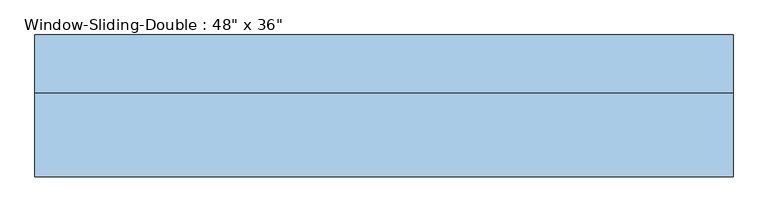
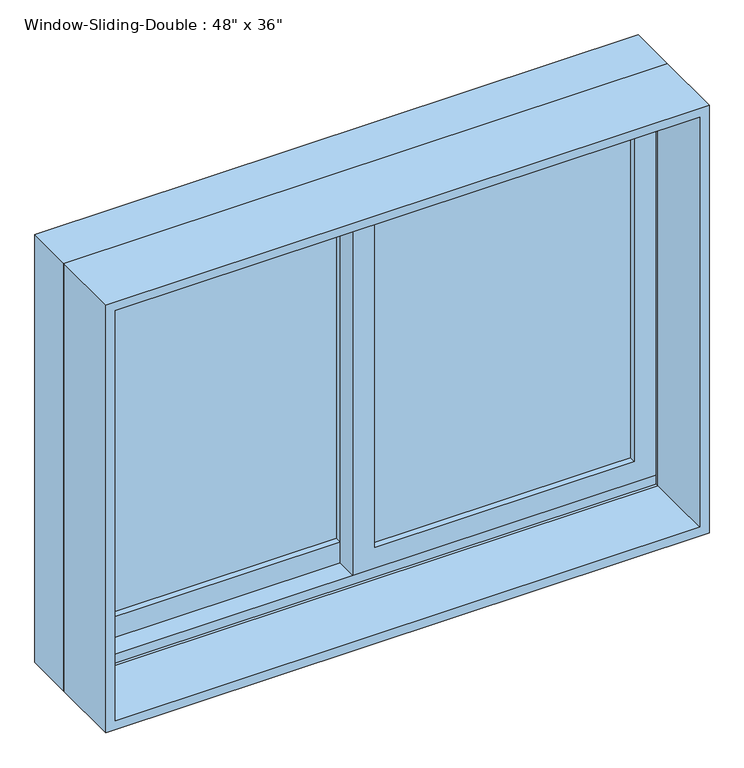
"""IFC4 building model written with IfcOpenShell, lengths in millimetres: window geometry."""

from ifc_helpers import new_model, si_unit, frame, origin, place, context, project, spatial, polyline, outline, extrude, faceted_brep, source, transform, mapped, element, save


def window_2eef0573(model_context):
    return source(origin(), model_context, "Body", "SolidModel", [
        extrude(outline(polyline([(952.5, 590.55), (1809.75, 590.55), (1809.75, -22.225), (952.5, -22.225), (952.5, 590.55)]), holes=[polyline([(996.95, 22.225), (1765.3, 22.225), (1765.3, 546.1), (996.95, 546.1), (996.95, 22.225)])]), frame((0.0, 34.29, 0.0), z_axis=(0.0, 1.0, 0.0), x_axis=(0.0, 0.0, 1.0)), (0.0, 0.0, 1.0), 44.45),
        extrude(outline(polyline([(933.45, -590.55), (933.45, 22.225), (1809.75, 22.225), (1809.75, -590.55), (933.45, -590.55)]), holes=[polyline([(1765.3, -22.225), (996.95, -22.225), (996.95, -546.1), (1765.3, -546.1), (1765.3, -22.225)])]), frame((0.0, 78.74, 0.0), z_axis=(0.0, 1.0, 0.0), x_axis=(0.0, 0.0, 1.0)), (0.0, 0.0, 1.0), 44.45),
        extrude(outline(polyline([(-22.225, 110.49), (-22.225, 104.14), (-546.1, 104.14), (-546.1, 110.49), (-22.225, 110.49)])), frame((0.0, 0.0, 996.95), z_axis=(0.0, 0.0, 1.0), x_axis=(1.0, 0.0, 0.0)), (0.0, 0.0, 1.0), 768.35),
        extrude(outline(polyline([(-22.225, 97.79), (-22.225, 91.44), (-546.1, 91.44), (-546.1, 97.79), (-22.225, 97.79)])), frame((0.0, 0.0, 996.95), z_axis=(0.0, 0.0, 1.0), x_axis=(1.0, 0.0, 0.0)), (0.0, 0.0, 1.0), 768.35),
        extrude(outline(polyline([(546.1, 66.04), (546.1, 59.69), (22.225, 59.69), (22.225, 66.04), (546.1, 66.04)])), frame((0.0, 0.0, 996.95), z_axis=(0.0, 0.0, 1.0), x_axis=(1.0, 0.0, 0.0)), (0.0, 0.0, 1.0), 768.35),
        extrude(outline(polyline([(546.1, 53.34), (546.1, 46.99), (22.225, 46.99), (22.225, 53.34), (546.1, 53.34)])), frame((0.0, 0.0, 996.95), z_axis=(0.0, 0.0, 1.0), x_axis=(1.0, 0.0, 0.0)), (0.0, 0.0, 1.0), 768.35),
        extrude(outline(polyline([(1828.8, -609.6), (914.4, -609.6), (914.4, 609.6), (1828.8, 609.6), (1828.8, -609.6)]), holes=[polyline([(1809.75, 590.55), (933.45, 590.55), (933.45, -590.55), (1809.75, -590.55), (1809.75, 590.55)])]), frame((0.0, -118.11, 0.0), z_axis=(0.0, 1.0, 0.0), x_axis=(0.0, 0.0, 1.0)), (0.0, 0.0, 1.0), 146.05),
        faceted_brep([(-609.6, 27.94, 914.4), (-609.6, 129.54, 914.4), (609.6, 129.54, 914.4), (609.6, 27.94, 914.4), (-568.6778905, 129.54, 1787.8778905), (-568.6778905, 123.19, 1787.8778905), (-568.6778905, 123.19, 933.45), (-568.6778905, 129.54, 933.45), (568.6778905, 123.19, 1787.8778905), (568.6778905, 123.19, 933.45), (590.55, 123.19, 933.45), (590.55, 123.19, 1809.75), (-590.55, 123.19, 1809.75), (-590.55, 123.19, 933.45), (-590.55, 27.94, 1809.75), (-590.55, 27.94, 933.45), (-590.55, 34.29, 933.45), (-590.55, 34.29, 952.5), (-590.55, 78.74, 952.5), (-590.55, 78.74, 933.45), (609.6, 27.94, 1828.8), (-609.6, 27.94, 1828.8), (590.55, 27.94, 1809.75), (590.55, 27.94, 933.45), (-609.6, 129.54, 1828.8), (609.6, 129.54, 1828.8), (568.6778905, 129.54, 933.45), (568.6778905, 129.54, 1787.8778905), (590.55, 78.74, 933.45), (590.55, 78.74, 952.5), (590.55, 34.29, 952.5), (590.55, 34.29, 933.45)], [[[0, 1, 2, 3]], [[4, 5, 6, 7]], [[5, 8, 9, 10, 11, 12, 13, 6]], [[12, 14, 15, 16, 17, 18, 19, 13]], [[0, 3, 20, 21], [22, 23, 15, 14]], [[24, 1, 0, 21]], [[2, 1, 24, 25], [4, 7, 26, 27]], [[5, 4, 27, 8]], [[12, 11, 22, 14]], [[21, 20, 25, 24]], [[8, 27, 26, 9]], [[22, 11, 10, 28, 29, 30, 31, 23]], [[20, 3, 2, 25]], [[26, 7, 6, 13, 19, 28, 10, 9]], [[28, 19, 18, 29]], [[29, 18, 17, 30]], [[30, 17, 16, 31]], [[15, 23, 31, 16]]]),
    ])


if __name__ == "__main__":
    model = new_model("IFC4")
    model_context = context("Model", 3, world=origin())
    ifc_project = project(units=[si_unit("LENGTHUNIT", "METRE", prefix="MILLI")], contexts=[model_context])
    site = spatial("IfcSite", under=ifc_project)
    building = spatial("IfcBuilding", under=site)
    placement = place(None, origin())
    window_shape = window_2eef0573(model_context)
    element("IfcWindow", 1, ObjectType="Window-Sliding-Double : 48\" x 36\"", at=placement, inside=building, context=model_context, shape_type="MappedRepresentation", body=[
        mapped(window_shape, transform((0.0, 0.0, 0.0), x_axis=(1.0, 0.0, 0.0), y_axis=(0.0, 1.0, 0.0), z_axis=(0.0, 0.0, 1.0))),
    ])
    save(model, "model.ifc")

# Revit data of these elements
# Type "Window-Sliding-Double : 48\" x 36\""
#   Type Mark = "18"
#   Fire Rating = "0.5h"
#   Assembly Code = "B2020100"
#   Analytic Construction = "Double glazing - domestic"
#   Window Inset [instance default] = 0' - 0"
#   Wall Thickness [instance default] = 0' - 6"
#   Visual Light Transmittance = 0.81
#   Thermal Resistance (R) = 1.8146 (h·ft²·°F)/BTU
#   Solar Heat Gain Coefficient = 0.76
#   Muntin Width = 1' - 8 5/8"
#   Muntin Height = 2' - 6 1/4"
#   Interior Wall Closure [instance default] = 0' - 2 3/4"
#   Heat Transfer Coefficient (U) = 0.5511 BTU/(h·ft²·°F)
#   Frame Extension [instance default] = 0' - 0 1/4"
#   Exterior Wall Closure [instance default] = 0' - 1 1/4"
#   Rough Width = 4' - 0 1/2"
#   Rough Height = 3' - 0 1/2"
#   Height = 3' - 0"
#   Extension Jamb [instance default] = 0' - 2 3/4"
#   Default Sill Height = 3' - 0"
#   Width = 4' - 0"
#   Interior Trim Visibility [instance default] = yes
#   Indicator Visibility [instance default] = yes
#   Exterior Trim Visibility [instance default] = yes
#   Muntin Visibility = yes
#   Extension Jamb Visibility [instance default] = yes
#   Muntin Pattern = Muntin Pattern_2x2 : Muntin Pattern_2x2
#   Interior Trim Material = Wood - Stained
#   Interior Trim = Trim-Window-Interior-Flat : Picture Frame
#   Interior Frame Material = Wood - Stained
#   Glass Panel Material = Glass
#   Exterior Trim Material = Clad - White
#   Exterior Trim = Trim-Window-Exterior-Flat : with Sill
#   Exterior Frame Material = Clad - White
#   Wall Closure = (empty or 0)
# Element 1 (IfcWindow, "Window-Sliding-Double : 48\" x 36\"")
#   Wall Thickness = 0' - 9"
#   Extension Jamb = 0' - 5 3/4"
#   Materials on its faces: "Wood - Stained", "Glass", "Clad - White"
# Materials
#   "Wood - Stained": class "Wood", colour RGB 224 178 126, transparency 0, Cost = 0
#   "Glass": class "Glass", colour RGB 0 128 192, transparency 0.75, Description = "Soda Lime Glass", Cost = 0
#   "Clad - White": class "Wood", colour RGB 242 242 238, transparency 0, Cost = 0
